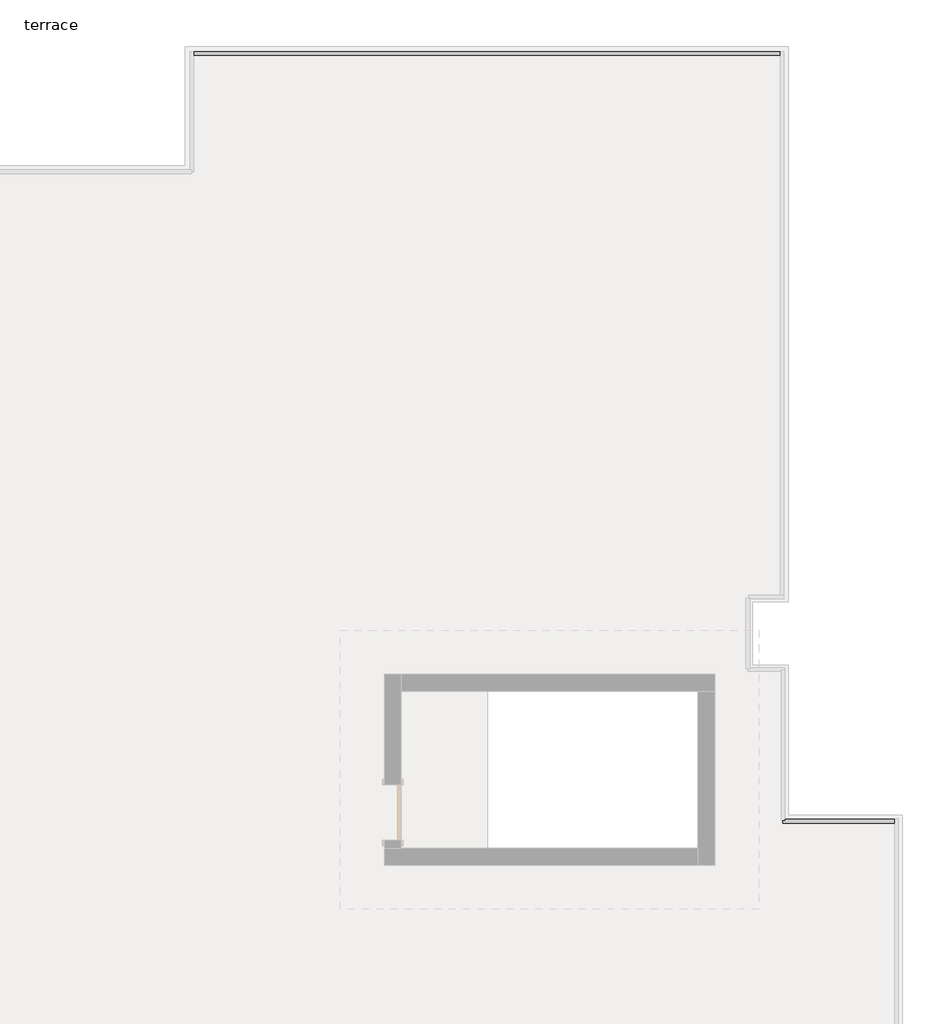
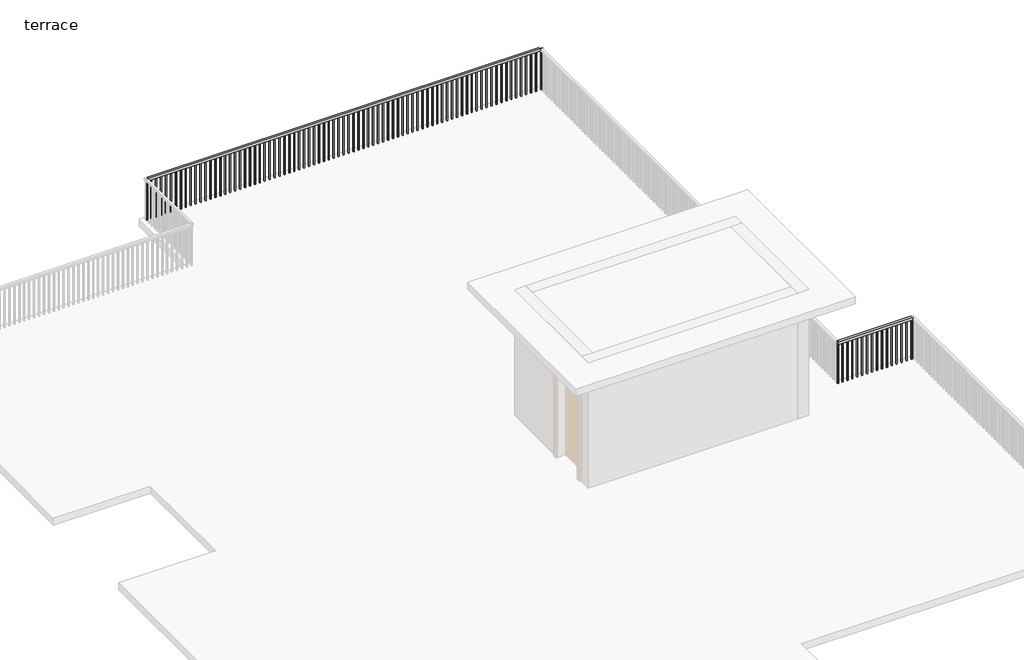
# One storey, part 7 of 7: 2 railings.
"""IFC4 building model written with IfcOpenShell, lengths in millimetres."""

from ifc_helpers import new_model, si_unit, frame, origin, place, context, project, spatial, polyline, outline, extrude, element, save

model = new_model("IFC4")

# Units and contexts
model_context = context("Model", 3, world=origin())
ifc_project = project(units=[si_unit("LENGTHUNIT", "METRE", prefix="MILLI")], contexts=[model_context])

# Site, building, storey
site = spatial("IfcSite", under=ifc_project)
building = spatial("IfcBuilding", under=site)
storey = spatial("IfcBuildingStorey", under=building, Name="terrace", Elevation=3810.0)

# Railings
placement = place(None, origin())
element("IfcRailing", 1, ObjectType="Handrail - Rectangular", at=placement, inside=storey, context=model_context, shape_type="SweptSolid", body=[
    extrude(outline(polyline([(-8409.8890129, 12608.227622), (-8409.8890129, 12659.027622), (-256.4890129, 12659.027622), (-256.4890129, 12608.227622), (-8409.8890129, 12608.227622)])), frame((0.0, 0.0, 4673.6), z_axis=(0.0, 0.0, 1.0), x_axis=(1.0, 0.0, 0.0)), (0.0, 0.0, 1.0), 50.8),
    extrude(outline(polyline([(-291.4140129, 12624.102622), (-291.4140129, 12643.152622), (-272.3640129, 12643.152622), (-272.3640129, 12624.102622), (-291.4140129, 12624.102622)])), frame((0.0, 0.0, 3810.0), z_axis=(0.0, 0.0, 1.0), x_axis=(1.0, 0.0, 0.0)), (0.0, 0.0, 1.0), 863.6),
    extrude(outline(polyline([(-393.0140129, 12624.102622), (-393.0140129, 12643.152622), (-373.9640129, 12643.152622), (-373.9640129, 12624.102622), (-393.0140129, 12624.102622)])), frame((0.0, 0.0, 3810.0), z_axis=(0.0, 0.0, 1.0), x_axis=(1.0, 0.0, 0.0)), (0.0, 0.0, 1.0), 863.6),
    extrude(outline(polyline([(-494.6140129, 12624.102622), (-494.6140129, 12643.152622), (-475.5640129, 12643.152622), (-475.5640129, 12624.102622), (-494.6140129, 12624.102622)])), frame((0.0, 0.0, 3810.0), z_axis=(0.0, 0.0, 1.0), x_axis=(1.0, 0.0, 0.0)), (0.0, 0.0, 1.0), 863.6),
    extrude(outline(polyline([(-596.2140129, 12624.102622), (-596.2140129, 12643.152622), (-577.1640129, 12643.152622), (-577.1640129, 12624.102622), (-596.2140129, 12624.102622)])), frame((0.0, 0.0, 3810.0), z_axis=(0.0, 0.0, 1.0), x_axis=(1.0, 0.0, 0.0)), (0.0, 0.0, 1.0), 863.6),
    extrude(outline(polyline([(-697.8140129, 12624.102622), (-697.8140129, 12643.152622), (-678.7640129, 12643.152622), (-678.7640129, 12624.102622), (-697.8140129, 12624.102622)])), frame((0.0, 0.0, 3810.0), z_axis=(0.0, 0.0, 1.0), x_axis=(1.0, 0.0, 0.0)), (0.0, 0.0, 1.0), 863.6),
    extrude(outline(polyline([(-799.4140129, 12624.102622), (-799.4140129, 12643.152622), (-780.3640129, 12643.152622), (-780.3640129, 12624.102622), (-799.4140129, 12624.102622)])), frame((0.0, 0.0, 3810.0), z_axis=(0.0, 0.0, 1.0), x_axis=(1.0, 0.0, 0.0)), (0.0, 0.0, 1.0), 863.6),
    extrude(outline(polyline([(-901.0140129, 12624.102622), (-901.0140129, 12643.152622), (-881.9640129, 12643.152622), (-881.9640129, 12624.102622), (-901.0140129, 12624.102622)])), frame((0.0, 0.0, 3810.0), z_axis=(0.0, 0.0, 1.0), x_axis=(1.0, 0.0, 0.0)), (0.0, 0.0, 1.0), 863.6),
    extrude(outline(polyline([(-1002.6140129, 12624.102622), (-1002.6140129, 12643.152622), (-983.5640129, 12643.152622), (-983.5640129, 12624.102622), (-1002.6140129, 12624.102622)])), frame((0.0, 0.0, 3810.0), z_axis=(0.0, 0.0, 1.0), x_axis=(1.0, 0.0, 0.0)), (0.0, 0.0, 1.0), 863.6),
    extrude(outline(polyline([(-1104.2140129, 12624.102622), (-1104.2140129, 12643.152622), (-1085.1640129, 12643.152622), (-1085.1640129, 12624.102622), (-1104.2140129, 12624.102622)])), frame((0.0, 0.0, 3810.0), z_axis=(0.0, 0.0, 1.0), x_axis=(1.0, 0.0, 0.0)), (0.0, 0.0, 1.0), 863.6),
    extrude(outline(polyline([(-1205.8140129, 12624.102622), (-1205.8140129, 12643.152622), (-1186.7640129, 12643.152622), (-1186.7640129, 12624.102622), (-1205.8140129, 12624.102622)])), frame((0.0, 0.0, 3810.0), z_axis=(0.0, 0.0, 1.0), x_axis=(1.0, 0.0, 0.0)), (0.0, 0.0, 1.0), 863.6),
    extrude(outline(polyline([(-1307.4140129, 12624.102622), (-1307.4140129, 12643.152622), (-1288.3640129, 12643.152622), (-1288.3640129, 12624.102622), (-1307.4140129, 12624.102622)])), frame((0.0, 0.0, 3810.0), z_axis=(0.0, 0.0, 1.0), x_axis=(1.0, 0.0, 0.0)), (0.0, 0.0, 1.0), 863.6),
    extrude(outline(polyline([(-1409.0140129, 12624.102622), (-1409.0140129, 12643.152622), (-1389.9640129, 12643.152622), (-1389.9640129, 12624.102622), (-1409.0140129, 12624.102622)])), frame((0.0, 0.0, 3810.0), z_axis=(0.0, 0.0, 1.0), x_axis=(1.0, 0.0, 0.0)), (0.0, 0.0, 1.0), 863.6),
    extrude(outline(polyline([(-1510.6140129, 12624.102622), (-1510.6140129, 12643.152622), (-1491.5640129, 12643.152622), (-1491.5640129, 12624.102622), (-1510.6140129, 12624.102622)])), frame((0.0, 0.0, 3810.0), z_axis=(0.0, 0.0, 1.0), x_axis=(1.0, 0.0, 0.0)), (0.0, 0.0, 1.0), 863.6),
    extrude(outline(polyline([(-1612.2140129, 12624.102622), (-1612.2140129, 12643.152622), (-1593.1640129, 12643.152622), (-1593.1640129, 12624.102622), (-1612.2140129, 12624.102622)])), frame((0.0, 0.0, 3810.0), z_axis=(0.0, 0.0, 1.0), x_axis=(1.0, 0.0, 0.0)), (0.0, 0.0, 1.0), 863.6),
    extrude(outline(polyline([(-1713.8140129, 12624.102622), (-1713.8140129, 12643.152622), (-1694.7640129, 12643.152622), (-1694.7640129, 12624.102622), (-1713.8140129, 12624.102622)])), frame((0.0, 0.0, 3810.0), z_axis=(0.0, 0.0, 1.0), x_axis=(1.0, 0.0, 0.0)), (0.0, 0.0, 1.0), 863.6),
    extrude(outline(polyline([(-1815.4140129, 12624.102622), (-1815.4140129, 12643.152622), (-1796.3640129, 12643.152622), (-1796.3640129, 12624.102622), (-1815.4140129, 12624.102622)])), frame((0.0, 0.0, 3810.0), z_axis=(0.0, 0.0, 1.0), x_axis=(1.0, 0.0, 0.0)), (0.0, 0.0, 1.0), 863.6),
    extrude(outline(polyline([(-1917.0140129, 12624.102622), (-1917.0140129, 12643.152622), (-1897.9640129, 12643.152622), (-1897.9640129, 12624.102622), (-1917.0140129, 12624.102622)])), frame((0.0, 0.0, 3810.0), z_axis=(0.0, 0.0, 1.0), x_axis=(1.0, 0.0, 0.0)), (0.0, 0.0, 1.0), 863.6),
    extrude(outline(polyline([(-2018.6140129, 12624.102622), (-2018.6140129, 12643.152622), (-1999.5640129, 12643.152622), (-1999.5640129, 12624.102622), (-2018.6140129, 12624.102622)])), frame((0.0, 0.0, 3810.0), z_axis=(0.0, 0.0, 1.0), x_axis=(1.0, 0.0, 0.0)), (0.0, 0.0, 1.0), 863.6),
    extrude(outline(polyline([(-2120.2140129, 12624.102622), (-2120.2140129, 12643.152622), (-2101.1640129, 12643.152622), (-2101.1640129, 12624.102622), (-2120.2140129, 12624.102622)])), frame((0.0, 0.0, 3810.0), z_axis=(0.0, 0.0, 1.0), x_axis=(1.0, 0.0, 0.0)), (0.0, 0.0, 1.0), 863.6),
    extrude(outline(polyline([(-2221.8140129, 12624.102622), (-2221.8140129, 12643.152622), (-2202.7640129, 12643.152622), (-2202.7640129, 12624.102622), (-2221.8140129, 12624.102622)])), frame((0.0, 0.0, 3810.0), z_axis=(0.0, 0.0, 1.0), x_axis=(1.0, 0.0, 0.0)), (0.0, 0.0, 1.0), 863.6),
    extrude(outline(polyline([(-2323.4140129, 12624.102622), (-2323.4140129, 12643.152622), (-2304.3640129, 12643.152622), (-2304.3640129, 12624.102622), (-2323.4140129, 12624.102622)])), frame((0.0, 0.0, 3810.0), z_axis=(0.0, 0.0, 1.0), x_axis=(1.0, 0.0, 0.0)), (0.0, 0.0, 1.0), 863.6),
    extrude(outline(polyline([(-2425.0140129, 12624.102622), (-2425.0140129, 12643.152622), (-2405.9640129, 12643.152622), (-2405.9640129, 12624.102622), (-2425.0140129, 12624.102622)])), frame((0.0, 0.0, 3810.0), z_axis=(0.0, 0.0, 1.0), x_axis=(1.0, 0.0, 0.0)), (0.0, 0.0, 1.0), 863.6),
    extrude(outline(polyline([(-2526.6140129, 12624.102622), (-2526.6140129, 12643.152622), (-2507.5640129, 12643.152622), (-2507.5640129, 12624.102622), (-2526.6140129, 12624.102622)])), frame((0.0, 0.0, 3810.0), z_axis=(0.0, 0.0, 1.0), x_axis=(1.0, 0.0, 0.0)), (0.0, 0.0, 1.0), 863.6),
    extrude(outline(polyline([(-2628.2140129, 12624.102622), (-2628.2140129, 12643.152622), (-2609.1640129, 12643.152622), (-2609.1640129, 12624.102622), (-2628.2140129, 12624.102622)])), frame((0.0, 0.0, 3810.0), z_axis=(0.0, 0.0, 1.0), x_axis=(1.0, 0.0, 0.0)), (0.0, 0.0, 1.0), 863.6),
    extrude(outline(polyline([(-2729.8140129, 12624.102622), (-2729.8140129, 12643.152622), (-2710.7640129, 12643.152622), (-2710.7640129, 12624.102622), (-2729.8140129, 12624.102622)])), frame((0.0, 0.0, 3810.0), z_axis=(0.0, 0.0, 1.0), x_axis=(1.0, 0.0, 0.0)), (0.0, 0.0, 1.0), 863.6),
    extrude(outline(polyline([(-2831.4140129, 12624.102622), (-2831.4140129, 12643.152622), (-2812.3640129, 12643.152622), (-2812.3640129, 12624.102622), (-2831.4140129, 12624.102622)])), frame((0.0, 0.0, 3810.0), z_axis=(0.0, 0.0, 1.0), x_axis=(1.0, 0.0, 0.0)), (0.0, 0.0, 1.0), 863.6),
    extrude(outline(polyline([(-2933.0140129, 12624.102622), (-2933.0140129, 12643.152622), (-2913.9640129, 12643.152622), (-2913.9640129, 12624.102622), (-2933.0140129, 12624.102622)])), frame((0.0, 0.0, 3810.0), z_axis=(0.0, 0.0, 1.0), x_axis=(1.0, 0.0, 0.0)), (0.0, 0.0, 1.0), 863.6),
    extrude(outline(polyline([(-3034.6140129, 12624.102622), (-3034.6140129, 12643.152622), (-3015.5640129, 12643.152622), (-3015.5640129, 12624.102622), (-3034.6140129, 12624.102622)])), frame((0.0, 0.0, 3810.0), z_axis=(0.0, 0.0, 1.0), x_axis=(1.0, 0.0, 0.0)), (0.0, 0.0, 1.0), 863.6),
    extrude(outline(polyline([(-3136.2140129, 12624.102622), (-3136.2140129, 12643.152622), (-3117.1640129, 12643.152622), (-3117.1640129, 12624.102622), (-3136.2140129, 12624.102622)])), frame((0.0, 0.0, 3810.0), z_axis=(0.0, 0.0, 1.0), x_axis=(1.0, 0.0, 0.0)), (0.0, 0.0, 1.0), 863.6),
    extrude(outline(polyline([(-3237.8140129, 12624.102622), (-3237.8140129, 12643.152622), (-3218.7640129, 12643.152622), (-3218.7640129, 12624.102622), (-3237.8140129, 12624.102622)])), frame((0.0, 0.0, 3810.0), z_axis=(0.0, 0.0, 1.0), x_axis=(1.0, 0.0, 0.0)), (0.0, 0.0, 1.0), 863.6),
    extrude(outline(polyline([(-3339.4140129, 12624.102622), (-3339.4140129, 12643.152622), (-3320.3640129, 12643.152622), (-3320.3640129, 12624.102622), (-3339.4140129, 12624.102622)])), frame((0.0, 0.0, 3810.0), z_axis=(0.0, 0.0, 1.0), x_axis=(1.0, 0.0, 0.0)), (0.0, 0.0, 1.0), 863.6),
    extrude(outline(polyline([(-3441.0140129, 12624.102622), (-3441.0140129, 12643.152622), (-3421.9640129, 12643.152622), (-3421.9640129, 12624.102622), (-3441.0140129, 12624.102622)])), frame((0.0, 0.0, 3810.0), z_axis=(0.0, 0.0, 1.0), x_axis=(1.0, 0.0, 0.0)), (0.0, 0.0, 1.0), 863.6),
    extrude(outline(polyline([(-3542.6140129, 12624.102622), (-3542.6140129, 12643.152622), (-3523.5640129, 12643.152622), (-3523.5640129, 12624.102622), (-3542.6140129, 12624.102622)])), frame((0.0, 0.0, 3810.0), z_axis=(0.0, 0.0, 1.0), x_axis=(1.0, 0.0, 0.0)), (0.0, 0.0, 1.0), 863.6),
    extrude(outline(polyline([(-3644.2140129, 12624.102622), (-3644.2140129, 12643.152622), (-3625.1640129, 12643.152622), (-3625.1640129, 12624.102622), (-3644.2140129, 12624.102622)])), frame((0.0, 0.0, 3810.0), z_axis=(0.0, 0.0, 1.0), x_axis=(1.0, 0.0, 0.0)), (0.0, 0.0, 1.0), 863.6),
    extrude(outline(polyline([(-3745.8140129, 12624.102622), (-3745.8140129, 12643.152622), (-3726.7640129, 12643.152622), (-3726.7640129, 12624.102622), (-3745.8140129, 12624.102622)])), frame((0.0, 0.0, 3810.0), z_axis=(0.0, 0.0, 1.0), x_axis=(1.0, 0.0, 0.0)), (0.0, 0.0, 1.0), 863.6),
    extrude(outline(polyline([(-3847.4140129, 12624.102622), (-3847.4140129, 12643.152622), (-3828.3640129, 12643.152622), (-3828.3640129, 12624.102622), (-3847.4140129, 12624.102622)])), frame((0.0, 0.0, 3810.0), z_axis=(0.0, 0.0, 1.0), x_axis=(1.0, 0.0, 0.0)), (0.0, 0.0, 1.0), 863.6),
    extrude(outline(polyline([(-3949.0140129, 12624.102622), (-3949.0140129, 12643.152622), (-3929.9640129, 12643.152622), (-3929.9640129, 12624.102622), (-3949.0140129, 12624.102622)])), frame((0.0, 0.0, 3810.0), z_axis=(0.0, 0.0, 1.0), x_axis=(1.0, 0.0, 0.0)), (0.0, 0.0, 1.0), 863.6),
    extrude(outline(polyline([(-4050.6140129, 12624.102622), (-4050.6140129, 12643.152622), (-4031.5640129, 12643.152622), (-4031.5640129, 12624.102622), (-4050.6140129, 12624.102622)])), frame((0.0, 0.0, 3810.0), z_axis=(0.0, 0.0, 1.0), x_axis=(1.0, 0.0, 0.0)), (0.0, 0.0, 1.0), 863.6),
    extrude(outline(polyline([(-4152.2140129, 12624.102622), (-4152.2140129, 12643.152622), (-4133.1640129, 12643.152622), (-4133.1640129, 12624.102622), (-4152.2140129, 12624.102622)])), frame((0.0, 0.0, 3810.0), z_axis=(0.0, 0.0, 1.0), x_axis=(1.0, 0.0, 0.0)), (0.0, 0.0, 1.0), 863.6),
    extrude(outline(polyline([(-4253.8140129, 12624.102622), (-4253.8140129, 12643.152622), (-4234.7640129, 12643.152622), (-4234.7640129, 12624.102622), (-4253.8140129, 12624.102622)])), frame((0.0, 0.0, 3810.0), z_axis=(0.0, 0.0, 1.0), x_axis=(1.0, 0.0, 0.0)), (0.0, 0.0, 1.0), 863.6),
    extrude(outline(polyline([(-4355.4140129, 12624.102622), (-4355.4140129, 12643.152622), (-4336.3640129, 12643.152622), (-4336.3640129, 12624.102622), (-4355.4140129, 12624.102622)])), frame((0.0, 0.0, 3810.0), z_axis=(0.0, 0.0, 1.0), x_axis=(1.0, 0.0, 0.0)), (0.0, 0.0, 1.0), 863.6),
    extrude(outline(polyline([(-4457.0140129, 12624.102622), (-4457.0140129, 12643.152622), (-4437.9640129, 12643.152622), (-4437.9640129, 12624.102622), (-4457.0140129, 12624.102622)])), frame((0.0, 0.0, 3810.0), z_axis=(0.0, 0.0, 1.0), x_axis=(1.0, 0.0, 0.0)), (0.0, 0.0, 1.0), 863.6),
    extrude(outline(polyline([(-4558.6140129, 12624.102622), (-4558.6140129, 12643.152622), (-4539.5640129, 12643.152622), (-4539.5640129, 12624.102622), (-4558.6140129, 12624.102622)])), frame((0.0, 0.0, 3810.0), z_axis=(0.0, 0.0, 1.0), x_axis=(1.0, 0.0, 0.0)), (0.0, 0.0, 1.0), 863.6),
    extrude(outline(polyline([(-4660.2140129, 12624.102622), (-4660.2140129, 12643.152622), (-4641.1640129, 12643.152622), (-4641.1640129, 12624.102622), (-4660.2140129, 12624.102622)])), frame((0.0, 0.0, 3810.0), z_axis=(0.0, 0.0, 1.0), x_axis=(1.0, 0.0, 0.0)), (0.0, 0.0, 1.0), 863.6),
    extrude(outline(polyline([(-4761.8140129, 12624.102622), (-4761.8140129, 12643.152622), (-4742.7640129, 12643.152622), (-4742.7640129, 12624.102622), (-4761.8140129, 12624.102622)])), frame((0.0, 0.0, 3810.0), z_axis=(0.0, 0.0, 1.0), x_axis=(1.0, 0.0, 0.0)), (0.0, 0.0, 1.0), 863.6),
    extrude(outline(polyline([(-4863.4140129, 12624.102622), (-4863.4140129, 12643.152622), (-4844.3640129, 12643.152622), (-4844.3640129, 12624.102622), (-4863.4140129, 12624.102622)])), frame((0.0, 0.0, 3810.0), z_axis=(0.0, 0.0, 1.0), x_axis=(1.0, 0.0, 0.0)), (0.0, 0.0, 1.0), 863.6),
    extrude(outline(polyline([(-4965.0140129, 12624.102622), (-4965.0140129, 12643.152622), (-4945.9640129, 12643.152622), (-4945.9640129, 12624.102622), (-4965.0140129, 12624.102622)])), frame((0.0, 0.0, 3810.0), z_axis=(0.0, 0.0, 1.0), x_axis=(1.0, 0.0, 0.0)), (0.0, 0.0, 1.0), 863.6),
    extrude(outline(polyline([(-5066.6140129, 12624.102622), (-5066.6140129, 12643.152622), (-5047.5640129, 12643.152622), (-5047.5640129, 12624.102622), (-5066.6140129, 12624.102622)])), frame((0.0, 0.0, 3810.0), z_axis=(0.0, 0.0, 1.0), x_axis=(1.0, 0.0, 0.0)), (0.0, 0.0, 1.0), 863.6),
    extrude(outline(polyline([(-5168.2140129, 12624.102622), (-5168.2140129, 12643.152622), (-5149.1640129, 12643.152622), (-5149.1640129, 12624.102622), (-5168.2140129, 12624.102622)])), frame((0.0, 0.0, 3810.0), z_axis=(0.0, 0.0, 1.0), x_axis=(1.0, 0.0, 0.0)), (0.0, 0.0, 1.0), 863.6),
    extrude(outline(polyline([(-5269.8140129, 12624.102622), (-5269.8140129, 12643.152622), (-5250.7640129, 12643.152622), (-5250.7640129, 12624.102622), (-5269.8140129, 12624.102622)])), frame((0.0, 0.0, 3810.0), z_axis=(0.0, 0.0, 1.0), x_axis=(1.0, 0.0, 0.0)), (0.0, 0.0, 1.0), 863.6),
    extrude(outline(polyline([(-5371.4140129, 12624.102622), (-5371.4140129, 12643.152622), (-5352.3640129, 12643.152622), (-5352.3640129, 12624.102622), (-5371.4140129, 12624.102622)])), frame((0.0, 0.0, 3810.0), z_axis=(0.0, 0.0, 1.0), x_axis=(1.0, 0.0, 0.0)), (0.0, 0.0, 1.0), 863.6),
    extrude(outline(polyline([(-5473.0140129, 12624.102622), (-5473.0140129, 12643.152622), (-5453.9640129, 12643.152622), (-5453.9640129, 12624.102622), (-5473.0140129, 12624.102622)])), frame((0.0, 0.0, 3810.0), z_axis=(0.0, 0.0, 1.0), x_axis=(1.0, 0.0, 0.0)), (0.0, 0.0, 1.0), 863.6),
    extrude(outline(polyline([(-5574.6140129, 12624.102622), (-5574.6140129, 12643.152622), (-5555.5640129, 12643.152622), (-5555.5640129, 12624.102622), (-5574.6140129, 12624.102622)])), frame((0.0, 0.0, 3810.0), z_axis=(0.0, 0.0, 1.0), x_axis=(1.0, 0.0, 0.0)), (0.0, 0.0, 1.0), 863.6),
    extrude(outline(polyline([(-5676.2140129, 12624.102622), (-5676.2140129, 12643.152622), (-5657.1640129, 12643.152622), (-5657.1640129, 12624.102622), (-5676.2140129, 12624.102622)])), frame((0.0, 0.0, 3810.0), z_axis=(0.0, 0.0, 1.0), x_axis=(1.0, 0.0, 0.0)), (0.0, 0.0, 1.0), 863.6),
    extrude(outline(polyline([(-5777.8140129, 12624.102622), (-5777.8140129, 12643.152622), (-5758.7640129, 12643.152622), (-5758.7640129, 12624.102622), (-5777.8140129, 12624.102622)])), frame((0.0, 0.0, 3810.0), z_axis=(0.0, 0.0, 1.0), x_axis=(1.0, 0.0, 0.0)), (0.0, 0.0, 1.0), 863.6),
    extrude(outline(polyline([(-5879.4140129, 12624.102622), (-5879.4140129, 12643.152622), (-5860.3640129, 12643.152622), (-5860.3640129, 12624.102622), (-5879.4140129, 12624.102622)])), frame((0.0, 0.0, 3810.0), z_axis=(0.0, 0.0, 1.0), x_axis=(1.0, 0.0, 0.0)), (0.0, 0.0, 1.0), 863.6),
    extrude(outline(polyline([(-5981.0140129, 12624.102622), (-5981.0140129, 12643.152622), (-5961.9640129, 12643.152622), (-5961.9640129, 12624.102622), (-5981.0140129, 12624.102622)])), frame((0.0, 0.0, 3810.0), z_axis=(0.0, 0.0, 1.0), x_axis=(1.0, 0.0, 0.0)), (0.0, 0.0, 1.0), 863.6),
    extrude(outline(polyline([(-6082.6140129, 12624.102622), (-6082.6140129, 12643.152622), (-6063.5640129, 12643.152622), (-6063.5640129, 12624.102622), (-6082.6140129, 12624.102622)])), frame((0.0, 0.0, 3810.0), z_axis=(0.0, 0.0, 1.0), x_axis=(1.0, 0.0, 0.0)), (0.0, 0.0, 1.0), 863.6),
    extrude(outline(polyline([(-6184.2140129, 12624.102622), (-6184.2140129, 12643.152622), (-6165.1640129, 12643.152622), (-6165.1640129, 12624.102622), (-6184.2140129, 12624.102622)])), frame((0.0, 0.0, 3810.0), z_axis=(0.0, 0.0, 1.0), x_axis=(1.0, 0.0, 0.0)), (0.0, 0.0, 1.0), 863.6),
    extrude(outline(polyline([(-6285.8140129, 12624.102622), (-6285.8140129, 12643.152622), (-6266.7640129, 12643.152622), (-6266.7640129, 12624.102622), (-6285.8140129, 12624.102622)])), frame((0.0, 0.0, 3810.0), z_axis=(0.0, 0.0, 1.0), x_axis=(1.0, 0.0, 0.0)), (0.0, 0.0, 1.0), 863.6),
    extrude(outline(polyline([(-6387.4140129, 12624.102622), (-6387.4140129, 12643.152622), (-6368.3640129, 12643.152622), (-6368.3640129, 12624.102622), (-6387.4140129, 12624.102622)])), frame((0.0, 0.0, 3810.0), z_axis=(0.0, 0.0, 1.0), x_axis=(1.0, 0.0, 0.0)), (0.0, 0.0, 1.0), 863.6),
    extrude(outline(polyline([(-6489.0140129, 12624.102622), (-6489.0140129, 12643.152622), (-6469.9640129, 12643.152622), (-6469.9640129, 12624.102622), (-6489.0140129, 12624.102622)])), frame((0.0, 0.0, 3810.0), z_axis=(0.0, 0.0, 1.0), x_axis=(1.0, 0.0, 0.0)), (0.0, 0.0, 1.0), 863.6),
    extrude(outline(polyline([(-6590.6140129, 12624.102622), (-6590.6140129, 12643.152622), (-6571.5640129, 12643.152622), (-6571.5640129, 12624.102622), (-6590.6140129, 12624.102622)])), frame((0.0, 0.0, 3810.0), z_axis=(0.0, 0.0, 1.0), x_axis=(1.0, 0.0, 0.0)), (0.0, 0.0, 1.0), 863.6),
    extrude(outline(polyline([(-6692.2140129, 12624.102622), (-6692.2140129, 12643.152622), (-6673.1640129, 12643.152622), (-6673.1640129, 12624.102622), (-6692.2140129, 12624.102622)])), frame((0.0, 0.0, 3810.0), z_axis=(0.0, 0.0, 1.0), x_axis=(1.0, 0.0, 0.0)), (0.0, 0.0, 1.0), 863.6),
    extrude(outline(polyline([(-6793.8140129, 12624.102622), (-6793.8140129, 12643.152622), (-6774.7640129, 12643.152622), (-6774.7640129, 12624.102622), (-6793.8140129, 12624.102622)])), frame((0.0, 0.0, 3810.0), z_axis=(0.0, 0.0, 1.0), x_axis=(1.0, 0.0, 0.0)), (0.0, 0.0, 1.0), 863.6),
    extrude(outline(polyline([(-6895.4140129, 12624.102622), (-6895.4140129, 12643.152622), (-6876.3640129, 12643.152622), (-6876.3640129, 12624.102622), (-6895.4140129, 12624.102622)])), frame((0.0, 0.0, 3810.0), z_axis=(0.0, 0.0, 1.0), x_axis=(1.0, 0.0, 0.0)), (0.0, 0.0, 1.0), 863.6),
    extrude(outline(polyline([(-6997.0140129, 12624.102622), (-6997.0140129, 12643.152622), (-6977.9640129, 12643.152622), (-6977.9640129, 12624.102622), (-6997.0140129, 12624.102622)])), frame((0.0, 0.0, 3810.0), z_axis=(0.0, 0.0, 1.0), x_axis=(1.0, 0.0, 0.0)), (0.0, 0.0, 1.0), 863.6),
    extrude(outline(polyline([(-7098.6140129, 12624.102622), (-7098.6140129, 12643.152622), (-7079.5640129, 12643.152622), (-7079.5640129, 12624.102622), (-7098.6140129, 12624.102622)])), frame((0.0, 0.0, 3810.0), z_axis=(0.0, 0.0, 1.0), x_axis=(1.0, 0.0, 0.0)), (0.0, 0.0, 1.0), 863.6),
    extrude(outline(polyline([(-7200.2140129, 12624.102622), (-7200.2140129, 12643.152622), (-7181.1640129, 12643.152622), (-7181.1640129, 12624.102622), (-7200.2140129, 12624.102622)])), frame((0.0, 0.0, 3810.0), z_axis=(0.0, 0.0, 1.0), x_axis=(1.0, 0.0, 0.0)), (0.0, 0.0, 1.0), 863.6),
    extrude(outline(polyline([(-7301.8140129, 12624.102622), (-7301.8140129, 12643.152622), (-7282.7640129, 12643.152622), (-7282.7640129, 12624.102622), (-7301.8140129, 12624.102622)])), frame((0.0, 0.0, 3810.0), z_axis=(0.0, 0.0, 1.0), x_axis=(1.0, 0.0, 0.0)), (0.0, 0.0, 1.0), 863.6),
    extrude(outline(polyline([(-7403.4140129, 12624.102622), (-7403.4140129, 12643.152622), (-7384.3640129, 12643.152622), (-7384.3640129, 12624.102622), (-7403.4140129, 12624.102622)])), frame((0.0, 0.0, 3810.0), z_axis=(0.0, 0.0, 1.0), x_axis=(1.0, 0.0, 0.0)), (0.0, 0.0, 1.0), 863.6),
    extrude(outline(polyline([(-7505.0140129, 12624.102622), (-7505.0140129, 12643.152622), (-7485.9640129, 12643.152622), (-7485.9640129, 12624.102622), (-7505.0140129, 12624.102622)])), frame((0.0, 0.0, 3810.0), z_axis=(0.0, 0.0, 1.0), x_axis=(1.0, 0.0, 0.0)), (0.0, 0.0, 1.0), 863.6),
    extrude(outline(polyline([(-7606.6140129, 12624.102622), (-7606.6140129, 12643.152622), (-7587.5640129, 12643.152622), (-7587.5640129, 12624.102622), (-7606.6140129, 12624.102622)])), frame((0.0, 0.0, 3810.0), z_axis=(0.0, 0.0, 1.0), x_axis=(1.0, 0.0, 0.0)), (0.0, 0.0, 1.0), 863.6),
    extrude(outline(polyline([(-7708.2140129, 12624.102622), (-7708.2140129, 12643.152622), (-7689.1640129, 12643.152622), (-7689.1640129, 12624.102622), (-7708.2140129, 12624.102622)])), frame((0.0, 0.0, 3810.0), z_axis=(0.0, 0.0, 1.0), x_axis=(1.0, 0.0, 0.0)), (0.0, 0.0, 1.0), 863.6),
    extrude(outline(polyline([(-7809.8140129, 12624.102622), (-7809.8140129, 12643.152622), (-7790.7640129, 12643.152622), (-7790.7640129, 12624.102622), (-7809.8140129, 12624.102622)])), frame((0.0, 0.0, 3810.0), z_axis=(0.0, 0.0, 1.0), x_axis=(1.0, 0.0, 0.0)), (0.0, 0.0, 1.0), 863.6),
    extrude(outline(polyline([(-7911.4140129, 12624.102622), (-7911.4140129, 12643.152622), (-7892.3640129, 12643.152622), (-7892.3640129, 12624.102622), (-7911.4140129, 12624.102622)])), frame((0.0, 0.0, 3810.0), z_axis=(0.0, 0.0, 1.0), x_axis=(1.0, 0.0, 0.0)), (0.0, 0.0, 1.0), 863.6),
    extrude(outline(polyline([(-8013.0140129, 12624.102622), (-8013.0140129, 12643.152622), (-7993.9640129, 12643.152622), (-7993.9640129, 12624.102622), (-8013.0140129, 12624.102622)])), frame((0.0, 0.0, 3810.0), z_axis=(0.0, 0.0, 1.0), x_axis=(1.0, 0.0, 0.0)), (0.0, 0.0, 1.0), 863.6),
    extrude(outline(polyline([(-8114.6140129, 12624.102622), (-8114.6140129, 12643.152622), (-8095.5640129, 12643.152622), (-8095.5640129, 12624.102622), (-8114.6140129, 12624.102622)])), frame((0.0, 0.0, 3810.0), z_axis=(0.0, 0.0, 1.0), x_axis=(1.0, 0.0, 0.0)), (0.0, 0.0, 1.0), 863.6),
    extrude(outline(polyline([(-8216.2140129, 12624.102622), (-8216.2140129, 12643.152622), (-8197.1640129, 12643.152622), (-8197.1640129, 12624.102622), (-8216.2140129, 12624.102622)])), frame((0.0, 0.0, 3810.0), z_axis=(0.0, 0.0, 1.0), x_axis=(1.0, 0.0, 0.0)), (0.0, 0.0, 1.0), 863.6),
    extrude(outline(polyline([(-8317.8140129, 12624.102622), (-8317.8140129, 12643.152622), (-8298.7640129, 12643.152622), (-8298.7640129, 12624.102622), (-8317.8140129, 12624.102622)])), frame((0.0, 0.0, 3810.0), z_axis=(0.0, 0.0, 1.0), x_axis=(1.0, 0.0, 0.0)), (0.0, 0.0, 1.0), 863.6),
    extrude(outline(polyline([(-275.5390129, 12624.102622), (-275.5390129, 12643.152622), (-256.4890129, 12643.152622), (-256.4890129, 12624.102622), (-275.5390129, 12624.102622)])), frame((0.0, 0.0, 3810.0), z_axis=(0.0, 0.0, 1.0), x_axis=(1.0, 0.0, 0.0)), (0.0, 0.0, 1.0), 863.6),
    extrude(outline(polyline([(-8409.8890129, 12624.102622), (-8409.8890129, 12643.152622), (-8390.8390129, 12643.152622), (-8390.8390129, 12624.102622), (-8409.8890129, 12624.102622)])), frame((0.0, 0.0, 3810.0), z_axis=(0.0, 0.0, 1.0), x_axis=(1.0, 0.0, 0.0)), (0.0, 0.0, 1.0), 863.6),
])
element("IfcRailing", 2, ObjectType="Handrail - Rectangular", at=placement, inside=storey, context=model_context, shape_type="SweptSolid", body=[
    extrude(outline(polyline([(-269.1890129, 2041.827622), (-269.1890129, 2092.627622), (1280.2109871, 2092.627622), (1280.2109871, 2041.827622), (-269.1890129, 2041.827622)])), frame((0.0, 0.0, 4673.6), z_axis=(0.0, 0.0, 1.0), x_axis=(1.0, 0.0, 0.0)), (0.0, 0.0, 1.0), 50.8),
    extrude(outline(polyline([(1245.2859871, 2057.702622), (1245.2859871, 2076.752622), (1264.3359871, 2076.752622), (1264.3359871, 2057.702622), (1245.2859871, 2057.702622)])), frame((0.0, 0.0, 3810.0), z_axis=(0.0, 0.0, 1.0), x_axis=(1.0, 0.0, 0.0)), (0.0, 0.0, 1.0), 863.6),
    extrude(outline(polyline([(1143.6859871, 2057.702622), (1143.6859871, 2076.752622), (1162.7359871, 2076.752622), (1162.7359871, 2057.702622), (1143.6859871, 2057.702622)])), frame((0.0, 0.0, 3810.0), z_axis=(0.0, 0.0, 1.0), x_axis=(1.0, 0.0, 0.0)), (0.0, 0.0, 1.0), 863.6),
    extrude(outline(polyline([(1042.0859871, 2057.702622), (1042.0859871, 2076.752622), (1061.1359871, 2076.752622), (1061.1359871, 2057.702622), (1042.0859871, 2057.702622)])), frame((0.0, 0.0, 3810.0), z_axis=(0.0, 0.0, 1.0), x_axis=(1.0, 0.0, 0.0)), (0.0, 0.0, 1.0), 863.6),
    extrude(outline(polyline([(940.4859871, 2057.702622), (940.4859871, 2076.752622), (959.5359871, 2076.752622), (959.5359871, 2057.702622), (940.4859871, 2057.702622)])), frame((0.0, 0.0, 3810.0), z_axis=(0.0, 0.0, 1.0), x_axis=(1.0, 0.0, 0.0)), (0.0, 0.0, 1.0), 863.6),
    extrude(outline(polyline([(838.8859871, 2057.702622), (838.8859871, 2076.752622), (857.9359871, 2076.752622), (857.9359871, 2057.702622), (838.8859871, 2057.702622)])), frame((0.0, 0.0, 3810.0), z_axis=(0.0, 0.0, 1.0), x_axis=(1.0, 0.0, 0.0)), (0.0, 0.0, 1.0), 863.6),
    extrude(outline(polyline([(737.2859871, 2057.702622), (737.2859871, 2076.752622), (756.3359871, 2076.752622), (756.3359871, 2057.702622), (737.2859871, 2057.702622)])), frame((0.0, 0.0, 3810.0), z_axis=(0.0, 0.0, 1.0), x_axis=(1.0, 0.0, 0.0)), (0.0, 0.0, 1.0), 863.6),
    extrude(outline(polyline([(635.6859871, 2057.702622), (635.6859871, 2076.752622), (654.7359871, 2076.752622), (654.7359871, 2057.702622), (635.6859871, 2057.702622)])), frame((0.0, 0.0, 3810.0), z_axis=(0.0, 0.0, 1.0), x_axis=(1.0, 0.0, 0.0)), (0.0, 0.0, 1.0), 863.6),
    extrude(outline(polyline([(534.0859871, 2057.702622), (534.0859871, 2076.752622), (553.1359871, 2076.752622), (553.1359871, 2057.702622), (534.0859871, 2057.702622)])), frame((0.0, 0.0, 3810.0), z_axis=(0.0, 0.0, 1.0), x_axis=(1.0, 0.0, 0.0)), (0.0, 0.0, 1.0), 863.6),
    extrude(outline(polyline([(432.4859871, 2057.702622), (432.4859871, 2076.752622), (451.5359871, 2076.752622), (451.5359871, 2057.702622), (432.4859871, 2057.702622)])), frame((0.0, 0.0, 3810.0), z_axis=(0.0, 0.0, 1.0), x_axis=(1.0, 0.0, 0.0)), (0.0, 0.0, 1.0), 863.6),
    extrude(outline(polyline([(330.8859871, 2057.702622), (330.8859871, 2076.752622), (349.9359871, 2076.752622), (349.9359871, 2057.702622), (330.8859871, 2057.702622)])), frame((0.0, 0.0, 3810.0), z_axis=(0.0, 0.0, 1.0), x_axis=(1.0, 0.0, 0.0)), (0.0, 0.0, 1.0), 863.6),
    extrude(outline(polyline([(229.2859871, 2057.702622), (229.2859871, 2076.752622), (248.3359871, 2076.752622), (248.3359871, 2057.702622), (229.2859871, 2057.702622)])), frame((0.0, 0.0, 3810.0), z_axis=(0.0, 0.0, 1.0), x_axis=(1.0, 0.0, 0.0)), (0.0, 0.0, 1.0), 863.6),
    extrude(outline(polyline([(127.6859871, 2057.702622), (127.6859871, 2076.752622), (146.7359871, 2076.752622), (146.7359871, 2057.702622), (127.6859871, 2057.702622)])), frame((0.0, 0.0, 3810.0), z_axis=(0.0, 0.0, 1.0), x_axis=(1.0, 0.0, 0.0)), (0.0, 0.0, 1.0), 863.6),
    extrude(outline(polyline([(26.0859871, 2057.702622), (26.0859871, 2076.752622), (45.1359871, 2076.752622), (45.1359871, 2057.702622), (26.0859871, 2057.702622)])), frame((0.0, 0.0, 3810.0), z_axis=(0.0, 0.0, 1.0), x_axis=(1.0, 0.0, 0.0)), (0.0, 0.0, 1.0), 863.6),
    extrude(outline(polyline([(-75.5140129, 2057.702622), (-75.5140129, 2076.752622), (-56.4640129, 2076.752622), (-56.4640129, 2057.702622), (-75.5140129, 2057.702622)])), frame((0.0, 0.0, 3810.0), z_axis=(0.0, 0.0, 1.0), x_axis=(1.0, 0.0, 0.0)), (0.0, 0.0, 1.0), 863.6),
    extrude(outline(polyline([(-177.1140129, 2057.702622), (-177.1140129, 2076.752622), (-158.0640129, 2076.752622), (-158.0640129, 2057.702622), (-177.1140129, 2057.702622)])), frame((0.0, 0.0, 3810.0), z_axis=(0.0, 0.0, 1.0), x_axis=(1.0, 0.0, 0.0)), (0.0, 0.0, 1.0), 863.6),
    extrude(outline(polyline([(1261.1609871, 2057.702622), (1261.1609871, 2076.752622), (1280.2109871, 2076.752622), (1280.2109871, 2057.702622), (1261.1609871, 2057.702622)])), frame((0.0, 0.0, 3810.0), z_axis=(0.0, 0.0, 1.0), x_axis=(1.0, 0.0, 0.0)), (0.0, 0.0, 1.0), 863.6),
    extrude(outline(polyline([(-269.1890129, 2057.702622), (-269.1890129, 2076.752622), (-250.1390129, 2076.752622), (-250.1390129, 2057.702622), (-269.1890129, 2057.702622)])), frame((0.0, 0.0, 3810.0), z_axis=(0.0, 0.0, 1.0), x_axis=(1.0, 0.0, 0.0)), (0.0, 0.0, 1.0), 863.6),
])

save(model, "model.ifc")

# Revit data of these elements
# Type "Handrail - Rectangular"
#   Assembly Code = "C2010400"
#   built-in parameter 1008612 = 0.0416667 (stored number, unit not read)
#   built-in parameter 1008611 = 0.0416667 (stored number, unit not read)
#   built-in parameter 1008609 = 0.333333 (stored number, unit not read)
#   built-in parameter 1008604 = 0.166667 (stored number, unit not read)
#   built-in parameter 1008603 = 0.166667 (stored number, unit not read)
#   Railing Height = 3' - 0"
#   built-in parameter 1008630 = 2
#   built-in parameter 1008610 = 2
#   built-in parameter 1008618 = Baluster - Square : 3/4"
# Elements 1, 2 (IfcRailing, "Handrail - Rectangular")
#   Phase Created = New Construction
